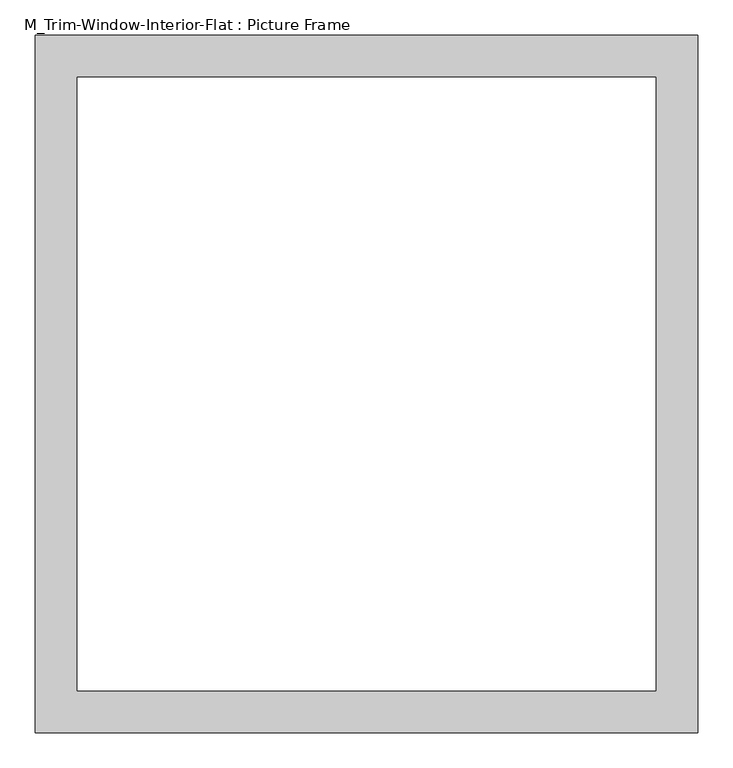
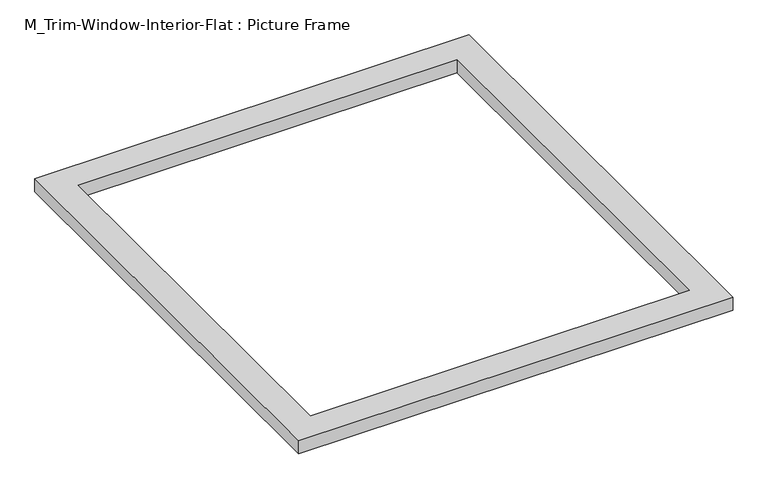
"""IFC4 building model written with IfcOpenShell, lengths in millimetres: proxy geometry, M_Trim-Window-Interior-Flat : Picture Frame."""

from ifc_helpers import new_model, si_unit, origin, origin_with_axes, place, context, project, spatial, polyline, outline, extrude, source, transform, mapped, element, save


def m_trim_window_interior_flat_picture_frame_6ca9b1f8(model_context):
    return source(origin(), model_context, "Body", "SweptSolid", [
        extrude(outline(polyline([(472.3, 47.3), (472.3, -947.3), (-472.3, -947.3), (-472.3, 47.3), (472.3, 47.3)]), holes=[polyline([(412.3, -12.7), (-412.3, -12.7), (-412.3, -887.3), (412.3, -887.3), (412.3, -12.7)])]), origin_with_axes(), (0.0, 0.0, 1.0), 30.0),
    ])


if __name__ == "__main__":
    model = new_model("IFC4")
    model_context = context("Model", 3, world=origin())
    ifc_project = project(units=[si_unit("LENGTHUNIT", "METRE", prefix="MILLI")], contexts=[model_context])
    site = spatial("IfcSite", under=ifc_project)
    building = spatial("IfcBuilding", under=site)
    placement = place(None, origin())
    m_trim_window_interior_flat_picture_frame_shape = m_trim_window_interior_flat_picture_frame_6ca9b1f8(model_context)
    element("IfcBuildingElementProxy", 1, Name="M_Trim-Window-Interior-Flat : Picture Frame", ObjectType="M_Trim-Window-Interior-Flat : Picture Frame", at=placement, inside=building, context=model_context, shape_type="MappedRepresentation", body=[
        mapped(m_trim_window_interior_flat_picture_frame_shape, transform((0.0, 0.0, 0.0), x_axis=(1.0, 0.0, 0.0), y_axis=(0.0, 1.0, 0.0), z_axis=(0.0, 0.0, 1.0))),
    ])
    save(model, "model.ifc")

# Revit data of these elements
# Type "M_Trim-Window-Interior-Flat : Picture Frame"
#   Trim Thickness_Picture Frame = 30 mm
#   Trim Width = 60 mm
#   Trim Thickness_with Sill = 20 mm
#   Sill Thickness = 30 mm
#   Opening Width [instance default] = 600 mm
#   Opening Height [instance default] = 900 mm
#   Default Elevation = 1200 mm
#   Sill = no
#   Picture Frame = yes
#   Trim Material [instance default] = none
# Element 1 (IfcBuildingElementProxy, "M_Trim-Window-Interior-Flat : Picture Frame")
#   Opening Width = 850 mm
#   Trim Material = Wood - Stained
#   Materials on its faces: "Wood - Stained"
# Materials
#   "Wood - Stained": class "Wood", colour RGB 224 178 126, transparency 0, Cost = 0
